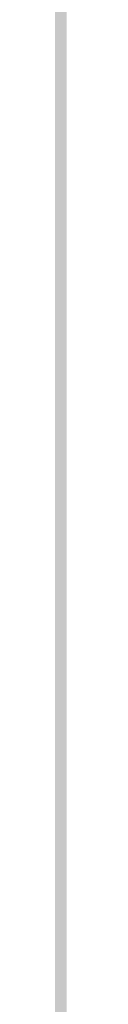
# Model space of a CAD drawing. Units: inches. Extents: x 2083 to 3317, y 1141 to 2115.
# Tile 201 of 256: x 3126.9579 to 3126.959, y 1263.6134 to 1264.1307. Entities that reach past the tile are written whole.
import ezdxf

# ---------------------------------------------------------------- set-up
doc = ezdxf.new("R2010")
doc.units = ezdxf.units.IN
doc.layers.add('A-ANNO-DIMS', color=2, linetype='Continuous', lineweight=18)
doc.layers.add('A-WALL-PATT', color=251, linetype='Continuous', lineweight=13, true_color=0x636466)
doc.styles.get("Standard").update_dxf_attribs({"font": 'arial.ttf'})
doc.dimstyles.new('ISO-25', dxfattribs={"dimtxt": 12, "dimasz": 12, "dimexe": 1.25, "dimexo": 0.625, "dimtad": 1, "dimlunit": 3, "dimtxsty": 'Standard', "dimcen": 2.5, "dimadec": 0, "dimazin": 0, "dimtfac": 1, "dimtmove": 0, "dimatfit": 3, "dimfxl": 1, "dimarcsym": 0})

# ---------------------------------------------------------------- blocks, each defined once
blk = doc.blocks.new('*D26')
at = {"layer": 'A-ANNO-DIMS', "color": 0, "lineweight": -2, "transparency": 16777216}
for p, q in [((3088.98584, 1274.91509), (3088.98584, 1270.95196)), ((3111.24004, 1274.91509), (3111.24004, 1270.95196)), ((3076.98584, 1272.20196), (2840.26245, 1272.20196)), ((3111.24004, 1272.20196), (3088.98584, 1272.20196)), ((3123.24004, 1272.20196), (3135.24004, 1272.20196))]:
    blk.add_line(p, q, dxfattribs=at)
at = {"layer": 'A-ANNO-DIMS', "color": 0, "transparency": 16777216}
for points in [[(3076.98584, 1274.20196), (3076.98584, 1270.20196), (3088.98584, 1272.20196)], [(3123.24004, 1274.20196), (3123.24004, 1270.20196), (3111.24004, 1272.20196)]]:
    blk.add_solid(points, dxfattribs=at)
at = {"layer": 'Defpoints', "color": 0, "transparency": 16777216}
for p in [(3088.98584, 1275.54009), (3111.24004, 1275.54009), (3088.98584, 1272.20196)]:
    blk.add_point(p, dxfattribs=at)
at = {"layer": 'A-ANNO-DIMS', "color": 0, "transparency": 16777216, "insert": (2952.62415, 1279.0316), "char_height": 12, "attachment_point": 5}
blk.add_mtext('NIGHTSTAND 1\'-10 1/2" TYP.', dxfattribs=at)
blk = doc.blocks.new('*D27')
at = {"layer": 'A-ANNO-DIMS', "color": 0, "lineweight": -2, "transparency": 16777216}
for p, q in [((3114.57817, 1309.79428), (3114.57817, 1321.79428)), ((3111.86504, 1297.79428), (3115.82817, 1297.79428)), ((3114.57817, 1297.79428), (3114.57817, 1275.54009)), ((3111.86504, 1275.54009), (3115.82817, 1275.54009)), ((3114.57817, 1263.54009), (3114.57817, 1140.98859))]:
    blk.add_line(p, q, dxfattribs=at)
at = {"layer": 'A-ANNO-DIMS', "color": 0, "transparency": 16777216}
for points in [[(3112.57817, 1309.79428), (3116.57817, 1309.79428), (3114.57817, 1297.79428)], [(3112.57817, 1263.54009), (3116.57817, 1263.54009), (3114.57817, 1275.54009)]]:
    blk.add_solid(points, dxfattribs=at)
at = {"layer": 'Defpoints', "color": 0, "transparency": 16777216}
for p in [(3111.24004, 1297.79428), (3111.24004, 1275.54009), (3114.57817, 1275.54009)]:
    blk.add_point(p, dxfattribs=at)
at = {"layer": 'A-ANNO-DIMS', "color": 0, "transparency": 16777216, "insert": (3107.74853, 1196.26434), "char_height": 12, "attachment_point": 5, "rotation": 90}
blk.add_mtext('1\'-10 1/2" TYP.', dxfattribs=at)

msp = doc.modelspace()

# ---------------------------------------------------------------- hatches: boundary and pattern name
at = {"layer": 'A-WALL-PATT'}
h = msp.add_hatch(color=256, dxfattribs=at)
h.dxf.hatch_style = 1
h.paths.add_polyline_path([(3126.95978, 2020.76136), (2748.95978, 2020.76136), (2604.95978, 2020.76136), (2226.95978, 2020.76136), (2226.95978, 1702.76136), (2466.95978, 1702.76136), (2466.95978, 1582.76136), (2418.95978, 1582.76136), (2418.95978, 1477.76136), (2226.95978, 1477.76136), (2226.95978, 1263.26136), (2544.95978, 1263.26136), (2544.95978, 1411.76136), (2604.95978, 1411.76136), (2685.95978, 1411.76136), (2685.95978, 1420.76136), (2604.95978, 1420.76136), (2604.95978, 1573.76136), (2604.95978, 1702.76136), (2604.95978, 2011.76136), (2748.95978, 2011.76136), (2748.95978, 1702.76136), (2862.95978, 1702.76136), (2862.95978, 1621.76136), (2871.95978, 1621.76136), (2871.95978, 1702.76136), (2883.95978, 1702.76136), (2883.95978, 1706.93946, -0.026459), (2883.95978, 1711.76136), (2757.95978, 1711.76136), (2757.95978, 1807.76136), (2787.95978, 1807.76136), (2787.95978, 1812.26136), (2757.95978, 1812.26136), (2757.95978, 2011.76136), (2877.95978, 2011.76136), (2877.95978, 1812.26136), (2847.95978, 1812.26136), (2847.95978, 1807.76136), (2889.83574, 1807.76136), (2889.83574, 1812.26136), (2882.45978, 1812.26136), (2882.45978, 2011.76136), (3117.95978, 2011.76136), (3117.95978, 1812.26136), (2937.83574, 1812.26136), (2937.83574, 1807.76136), (2995.70978, 1807.76136), (2995.70978, 1796.11767), (3000.20978, 1796.11767), (3000.20978, 1807.76136), (3117.95978, 1807.76136), (3117.95978, 1711.76136), (3000.20978, 1711.76136), (3000.20978, 1760.11767), (2998.5727, 1760.11767, -0.020711), (2995.70978, 1760.11767), (2995.70978, 1711.76136), (2931.95978, 1711.76136), (2931.95978, 1702.76136), (3126.95978, 1702.76136)])
h.paths.add_polyline_path([(2471.45978, 2011.76136), (2471.45978, 1810.01136), (2462.71694, 1810.01136), (2462.71694, 1805.51136), (2505.95978, 1805.51136), (2505.95978, 1810.01136), (2475.95978, 1810.01136), (2475.95978, 2011.76136), (2595.95978, 2011.76136), (2595.95978, 1810.01136), (2565.95978, 1810.01136), (2565.95978, 1805.51136), (2595.95978, 1805.51136), (2595.95978, 1711.76136), (2235.95978, 1711.76136), (2235.95978, 1805.51136), (2353.70978, 1805.51136), (2353.70978, 1796.05416), (2358.20978, 1796.05416), (2358.20978, 1805.51136), (2414.71694, 1805.51136), (2414.71694, 1810.01136), (2235.95978, 1810.01136), (2235.95978, 2011.76136)], flags=16)
h.paths.add_polyline_path([(2270.20473, 1994.61001), (2270.20473, 1970.61001), (2246.20473, 1970.61001), (2246.20473, 1994.61001)], flags=0)
edge = h.paths.add_edge_path(flags=0)
edge.add_ellipse((2332.02739, 1899.79818), major_axis=(-3.04299, 3.04299), ratio=0.1682525, start_angle=-161.33217, end_angle=-156.30711, ccw=False)
edge.add_ellipse((2333.08204, 1898.74353), major_axis=(-1.05465, 1.05465), ratio=0.4535321, start_angle=-123.37102, end_angle=-94.15911)
edge = h.paths.add_edge_path(flags=0)
edge.add_ellipse((2332.02739, 1968.87629), major_axis=(3.04299, 3.04299), ratio=0.1682525, start_angle=18.66783, end_angle=23.69289)
edge.add_spline(control_points=[(2332.9256, 1970.6911), (2332.22677, 1970.3361), (2330.89371, 1969.65891), (2328.41308, 1970.93214), (2327.20393, 1967.74871), (2324.7096, 1969.95559), (2322.53282, 1967.01235), (2320.01285, 1971.29581), (2317.68031, 1968.15784), (2316.04053, 1967.10205), (2315.4269, 1966.8096)], knot_values=[0, 0, 0, 0, 2.267059, 4.324559, 6.685584, 8.878641, 11.121502, 14.300359, 17.755284, 19.732645, 19.732645, 19.732645, 19.732645], degree=3, periodic=0)
edge.add_ellipse((2332.02739, 1968.87629), major_axis=(3.04299, 3.04299), ratio=0.1682525, start_angle=18.66783, end_angle=23.69289, ccw=False)
edge.add_ellipse((2333.08204, 1969.93094), major_axis=(1.05465, 1.05465), ratio=0.4535321, start_angle=56.62898, end_angle=85.84089, ccw=False)
edge = h.paths.add_edge_path(flags=0)
edge.add_spline(control_points=[(2296.42829, 1967.98791), (2293.6278, 1965.33631), (2287.70362, 1959.72709), (2299.74386, 1949.9957), (2294.53259, 1935.66853), (2290.57323, 1920.60351), (2293.39412, 1909.97369), (2296.18541, 1904.96654)], knot_values=[0.099185, 0.099185, 0.099185, 0.099185, 0.345301, 0.619822, 0.982653, 1.386093, 1.810555, 1.810555, 1.810555, 1.810555], degree=3, periodic=0)
edge.add_spline(control_points=[(2296.18541, 1904.96654), (2297.38358, 1902.6193), (2298.00097, 1901.94931), (2298.55297, 1901.46815)], knot_values=[0.006246, 0.006246, 0.006246, 0.006246, 0.055476, 0.055476, 0.055476, 0.055476], degree=3, periodic=0)
edge.add_spline(control_points=[(2298.55297, 1901.46815), (2297.25861, 1900.92322), (2295.22529, 1900.23213), (2293.06023, 1900.61421), (2292.10142, 1900.78841), (2292.08958, 1900.79057)], knot_values=[0.312835, 0.312835, 0.312835, 0.312835, 0.40178, 0.474987, 0.475903, 0.475903, 0.475903, 0.475903], degree=3, periodic=0)
edge.add_arc((2292.79365, 1904.66411), 3.93701, 215.4209, 259.69818, ccw=False)
edge.add_spline(control_points=[(2289.58531, 1902.3823), (2289.47665, 1902.53509), (2289.36848, 1902.68804), (2289.26086, 1902.84117)], knot_values=[0.102872, 0.102872, 0.102872, 0.102872, 0.116896, 0.116896, 0.116896, 0.116896], degree=3, periodic=0)
edge.add_spline(control_points=[(2289.26086, 1902.84117), (2288.6866, 1902.55019), (2287.64005, 1902.0199), (2285.88134, 1901.87395), (2283.85297, 1901.50435), (2281.71999, 1899.71054), (2278.46699, 1899.49294), (2276.15714, 1901.8832), (2272.25895, 1899.80407), (2267.77761, 1901.84318), (2262.24388, 1900.18403), (2257.41493, 1901.78206), (2254.31837, 1900.72612), (2253.17828, 1900.33734)], knot_values=[0, 0, 0, 0, 1.907977, 3.477176, 5.261074, 7.972851, 11.680248, 13.717921, 16.939592, 22.789562, 27.502503, 33.595215, 37.145618, 37.145618, 37.145618, 37.145618], degree=3, periodic=0)
edge.add_line((2253.17828, 1900.33734), (2250.24424, 1902.84117))
edge.add_line((2250.24424, 1902.84117), (2250.24424, 1965.8333))
edge.add_line((2250.24424, 1965.8333), (2253.17828, 1968.33712))
edge.add_spline(control_points=[(2253.17828, 1968.33712), (2254.31837, 1967.94835), (2257.41493, 1966.89241), (2262.24388, 1968.49043), (2267.77761, 1966.83128), (2271.52673, 1968.53722), (2273.87591, 1967.82829), (2274.2067, 1967.72764)], knot_values=[0, 0, 0, 0, 0.09018, 0.244935, 0.364644, 0.513233, 0.537855, 0.537855, 0.537855, 0.537855], degree=3, periodic=0)
edge.add_arc((2274.35289, 1963.79335), 3.93701, 72.05113, 92.12795, ccw=False)
edge.add_arc((2281.29693, 1985.23), 18.5963, 252.051134, 288.565722)
edge.add_arc((2292.31672, 1956.02888), 12.64608, 71.026788, 113.778218, ccw=False)
edge = h.paths.add_edge_path(flags=0)
edge.add_spline(control_points=[(2274.89941, 1951.85619), (2275.06616, 1951.61659), (2275.23269, 1951.37659), (2275.39799, 1951.13585)], knot_values=[1.409916, 1.409916, 1.409916, 1.409916, 1.43159, 1.43159, 1.43159, 1.43159], degree=3, periodic=0)
edge.add_spline(control_points=[(2275.39799, 1951.13585), (2275.79211, 1950.56189), (2276.17923, 1949.98377), (2276.54555, 1949.3971)], knot_values=[1.358238, 1.358238, 1.358238, 1.358238, 1.409916, 1.409916, 1.409916, 1.409916], degree=3, periodic=0)
edge.add_line((2276.54555, 1949.3971), (2277.43729, 1947.86218))
edge.add_spline(control_points=[(2277.43729, 1947.86218), (2276.30383, 1945.67311), (2274.6397, 1942.42688), (2274.63161, 1938.0939), (2272.79912, 1930.85155), (2274.35643, 1943.89705), (2275.94768, 1947.92336), (2276.54555, 1949.3971)], knot_values=[0.005632, 0.005632, 0.005632, 0.005632, 0.186014, 0.266002, 0.357087, 0.59639, 0.739732, 0.739732, 0.739732, 0.739732], degree=3, periodic=0)
edge.add_spline(control_points=[(2276.54555, 1949.3971), (2276.17923, 1949.98377), (2275.79211, 1950.56189), (2275.39799, 1951.13585)], knot_values=[1.358238, 1.358238, 1.358238, 1.358238, 1.409916, 1.409916, 1.409916, 1.409916], degree=3, periodic=0)
edge.add_spline(control_points=[(2275.39799, 1951.13585), (2274.9425, 1950.08045), (2274.20776, 1948.02527), (2273.9346, 1944.85148), (2272.46853, 1937.62749), (2273.46622, 1945.69647), (2274.70062, 1951.05947), (2274.89941, 1951.85619)], knot_values=[0.104364, 0.104364, 0.104364, 0.104364, 0.189636, 0.269624, 0.36071, 0.600013, 0.644622, 0.644622, 0.644622, 0.644622], degree=3, periodic=0)
h.paths.add_polyline_path([(2269.16751, 1963.12757, -0.357527), (2268.17063, 1960.97637, -0.092561), (2268.17063, 1939.43632, -0.357527), (2269.16751, 1937.28512, -0.357527), (2267.01631, 1938.282, -0.164785), (2254.68558, 1938.282, -0.357527), (2252.53438, 1937.28512, -0.357527), (2253.53126, 1939.43632, -0.092561), (2253.53126, 1960.97637, -0.357527), (2252.53438, 1963.12757, -0.357527), (2254.68558, 1962.13069, -0.164785), (2267.01631, 1962.13069, -0.357527)], flags=0)
h.paths.add_polyline_path([(2248.87407, 1967.8018), (2248.87407, 1957.02771), (2249.45778, 1957.02771), (2249.45778, 1911.64676), (2248.87407, 1911.64676), (2248.87407, 1900.87267), (2246.51186, 1900.87267, 0.197327), (2244.14966, 1902.45687), (2244.14966, 1966.21759, 0.197327), (2246.51186, 1967.8018)], flags=0)
h.paths.add_polyline_path([(2269.16751, 1931.38934, -0.357527), (2268.17063, 1929.23814, -0.092561), (2268.17063, 1907.6981, -0.357527), (2269.16751, 1905.54689, -0.357527), (2267.01631, 1906.54377, -0.164785), (2254.68558, 1906.54377, -0.357527), (2252.53438, 1905.54689, -0.357527), (2253.53126, 1907.6981, -0.092561), (2253.53126, 1929.23814, -0.357527), (2252.53438, 1931.38934, -0.357527), (2254.68558, 1930.39246, -0.164785), (2267.01631, 1930.39246, -0.357527)], flags=0)
edge = h.paths.add_edge_path(flags=0)
edge.add_spline(control_points=[(2276.19686, 1906.7237), (2276.16814, 1909.02893), (2276.11405, 1913.37185), (2270.59842, 1924.92498), (2273.90517, 1919.01278), (2275.92171, 1916.26206), (2275.47457, 1912.40215), (2277.25787, 1910.38062), (2276.69604, 1908.22504), (2276.64622, 1906.81302), (2276.61782, 1906.00841)], knot_values=[0, 0, 0, 0, 8.61026, 16.221274, 18.843057, 23.804898, 27.440828, 29.356102, 31.203478, 33.650687, 33.650687, 33.650687, 33.650687], degree=3, periodic=0)
edge.add_spline(control_points=[(2276.61782, 1906.00841), (2276.62331, 1905.62414), (2276.49774, 1904.62866), (2275.44178, 1903.85473), (2274.93731, 1903.08045), (2274.85908, 1902.84117)], knot_values=[0.156488, 0.156488, 0.156488, 0.156488, 0.184398, 0.231376, 0.250598, 0.250598, 0.250598, 0.250598], degree=3, periodic=0)
edge.add_line((2274.85908, 1902.84117), (2276.50598, 1902.84117))
edge.add_spline(control_points=[(2276.50598, 1902.84117), (2276.78831, 1903.08494), (2277.66507, 1904.1252), (2278.24954, 1904.34074), (2277.65387, 1908.52739), (2278.15567, 1906.22781), (2278.10046, 1905.28595), (2278.84667, 1904.06901), (2277.85679, 1903.41495), (2277.87419, 1902.99105), (2277.90356, 1902.84117)], knot_values=[0.059574, 0.059574, 0.059574, 0.059574, 0.080753, 0.103741, 0.16972, 0.176036, 0.207137, 0.240474, 0.262341, 0.27366, 0.27366, 0.27366, 0.27366], degree=3, periodic=0)
edge.add_line((2277.90356, 1902.84117), (2280.02983, 1902.84117))
edge.add_spline(control_points=[(2280.02983, 1902.84117), (2279.88822, 1903.0884), (2279.49926, 1903.98155), (2280.15228, 1905.93935), (2278.10362, 1909.65776), (2279.76239, 1907.18529), (2280.3279, 1904.87486), (2280.48511, 1903.48959), (2281.46327, 1903.24943), (2281.75834, 1902.9365), (2281.83404, 1902.84117)], knot_values=[0.013856, 0.013856, 0.013856, 0.013856, 0.034874, 0.088867, 0.107879, 0.126738, 0.158714, 0.193757, 0.217487, 0.226722, 0.226722, 0.226722, 0.226722], degree=3, periodic=0)
edge.add_spline(control_points=[(2281.83404, 1902.84117), (2281.78753, 1902.8267), (2281.64702, 1902.78299), (2281.39553, 1902.85949), (2281.08808, 1902.98524), (2280.72068, 1903.0609), (2280.33345, 1903.02573), (2280.12477, 1902.89888), (2280.02983, 1902.84117)], knot_values=[0, 0, 0, 0, 0.14413, 0.435517, 0.749276, 1.153046, 1.548371, 1.878348, 1.878348, 1.878348, 1.878348], degree=3, periodic=0)
edge.add_line((2280.02983, 1902.84117), (2277.90356, 1902.84117))
edge.add_spline(control_points=[(2277.90356, 1902.84117), (2277.89286, 1902.79586), (2277.8654, 1902.67964), (2277.60748, 1902.68748), (2277.27405, 1902.8007), (2276.83792, 1902.61977), (2276.58381, 1902.78926), (2276.50598, 1902.84117)], knot_values=[0, 0, 0, 0, 0.127189, 0.326199, 0.628009, 1.24357, 1.515331, 1.515331, 1.515331, 1.515331], degree=3, periodic=0)
edge.add_line((2276.50598, 1902.84117), (2274.85908, 1902.84117))
edge.add_spline(control_points=[(2274.85908, 1902.84117), (2274.81444, 1902.89859), (2274.72513, 1903.01345), (2274.49348, 1903.11897), (2274.24429, 1902.96054), (2273.93712, 1903.18494), (2273.61404, 1902.98314), (2273.40832, 1902.88304), (2273.32225, 1902.84117)], knot_values=[0, 0, 0, 0, 0.21843, 0.436957, 0.687977, 0.990379, 1.398396, 1.69185, 1.69185, 1.69185, 1.69185], degree=3, periodic=0)
edge.add_spline(control_points=[(2273.32225, 1902.84117), (2273.61674, 1903.44569), (2274.274, 1904.53825), (2276.02724, 1904.5737), (2276.20696, 1906.58364), (2276.19686, 1906.7237)], knot_values=[0.012227, 0.012227, 0.012227, 0.012227, 0.059472, 0.106218, 0.134458, 0.134458, 0.134458, 0.134458], degree=3, periodic=0)
h.paths.add_polyline_path([(2270.77605, 1897.78983), (2270.77605, 1873.78983), (2246.77605, 1873.78983), (2246.77605, 1897.78983)], flags=0)
h.paths.add_polyline_path([(2353.70978, 1760.00506), (2353.70978, 1760.05416), (2358.20978, 1760.05416, -0.033729)], flags=0)
h.paths.add_polyline_path([(2321.81912, 1737.52919), (2341.99533, 1737.52919, -0.414214), (2343.20327, 1736.32124), (2343.20327, 1721.0206, -0.414214), (2341.99533, 1719.81265), (2321.81912, 1719.81265, -0.414214), (2320.61117, 1721.0206), (2320.61117, 1736.32124, -0.414214)], flags=0)
h.paths.add_polyline_path([(2324.23501, 1736.32124), (2339.57944, 1736.32124, -0.414214), (2341.99533, 1733.90535), (2341.99533, 1725.44973, -0.414214), (2339.57944, 1723.03384), (2333.68059, 1723.03384), (2333.84532, 1722.04547, -0.870646), (2335.4254, 1721.82589, -0.767327), (2333.92269, 1721.42324), (2331.29102, 1721.42324, -0.767327), (2329.78832, 1721.82589, -0.870646), (2331.3684, 1722.04547), (2331.53313, 1723.03384), (2324.23501, 1723.03384, -0.414214), (2321.81912, 1725.44973), (2321.81912, 1733.90535, -0.414214)], flags=0)
h.paths.add_polyline_path([(2570.48379, 1928.61544), (2589.68379, 1928.61544), (2590.16883, 1928.61544), (2590.16883, 1904.9934), (2570.48379, 1904.9934)], flags=0)
h.paths.add_polyline_path([(2574.44732, 1927.26382, -1), (2572.82884, 1927.26382, -1)], flags=0)
h.paths.add_polyline_path([(2573.08987, 1926.94088), (2573.92503, 1927.77604), (2574.14774, 1927.55333), (2573.31258, 1926.71817)], flags=0)
h.paths.add_polyline_path([(2578.77906, 1919.72962, -1), (2571.59166, 1919.72962, -1)], flags=0)
h.paths.add_polyline_path([(2578.38536, 1919.72962, -1), (2571.98536, 1919.72962, -1)], flags=0)
h.paths.add_polyline_path([(2331.59576, 1729.47622, -1), (2333.61795, 1729.47622, -1)], flags=0)
h.paths.add_polyline_path([(2578.03423, 1927.26382, -1), (2576.41574, 1927.26382, -1)], flags=0)
h.paths.add_polyline_path([(2576.68885, 1927.53109), (2576.91156, 1927.7538), (2577.74673, 1926.91863), (2577.52402, 1926.69592)], flags=0)
h.paths.add_polyline_path([(2578.13906, 1909.85954, -1), (2572.23166, 1909.85954, -1)], flags=0)
h.paths.add_polyline_path([(2577.74536, 1909.85954, -1), (2572.62536, 1909.85954, -1)], flags=0)
h.paths.add_polyline_path([(2583.79772, 1927.26382, -1), (2582.17923, 1927.26382, -1)], flags=0)
h.paths.add_polyline_path([(2582.71865, 1927.7538), (2583.55381, 1926.91863), (2583.3311, 1926.69592), (2582.49594, 1927.53109)], flags=0)
h.paths.add_polyline_path([(2582.49594, 1927.53109), (2582.71865, 1927.7538), (2583.55381, 1926.91863), (2583.3311, 1926.69592)], flags=0)
h.paths.add_polyline_path([(2587.73906, 1920.52962, -1), (2581.83166, 1920.52962, -1)], flags=0)
h.paths.add_polyline_path([(2587.34536, 1920.52962, -1), (2582.22536, 1920.52962, -1)], flags=0)
h.paths.add_polyline_path([(2587.38462, 1927.26382, -1), (2585.76613, 1927.26382, -1)], flags=0)
h.paths.add_polyline_path([(2586.08199, 1926.98025), (2586.91716, 1927.81541), (2587.13987, 1927.5927), (2586.3047, 1926.75754)], flags=0)
h.paths.add_polyline_path([(2588.37906, 1910.65954, -1), (2581.19166, 1910.65954, -1)], flags=0)
h.paths.add_polyline_path([(2587.98536, 1910.65954, -1), (2581.58536, 1910.65954, -1)], flags=0)
h.paths.add_polyline_path([(2417.16773, 1729.4779), (2437.34394, 1729.4779, -0.414214), (2438.55188, 1728.26995), (2438.55188, 1712.96931, -0.414214), (2437.34394, 1711.76136), (2417.16773, 1711.76136, -0.414214), (2415.95978, 1712.96931), (2415.95978, 1728.26995, -0.414214)], flags=0)
h.paths.add_polyline_path([(2419.58362, 1728.26995), (2434.92805, 1728.26995, -0.414214), (2437.34394, 1725.85406), (2437.34394, 1717.39844, -0.414214), (2434.92805, 1714.98255), (2429.0292, 1714.98255), (2429.19393, 1713.99418, -0.870646), (2430.77401, 1713.7746, -0.767327), (2429.2713, 1713.37195), (2426.63963, 1713.37195, -0.767327), (2425.13693, 1713.7746, -0.870646), (2426.71701, 1713.99418), (2426.88174, 1714.98255), (2419.58362, 1714.98255, -0.414214), (2417.16773, 1717.39844), (2417.16773, 1725.85406, -0.414214)], flags=0)
h.paths.add_polyline_path([(2419.58362, 1728.26995), (2434.92805, 1728.26995, -0.414214), (2437.34394, 1725.85406), (2437.34394, 1717.39844, -0.414214), (2434.92805, 1714.98255), (2429.0292, 1714.98255), (2428.35812, 1719.00903), (2427.55282, 1719.00903), (2426.88174, 1714.98255), (2419.58362, 1714.98255, -0.414214), (2417.16773, 1717.39844), (2417.16773, 1725.85406, -0.414214)], flags=0)
h.paths.add_polyline_path([(2426.94437, 1721.42492, -1), (2428.96656, 1721.42492, -1)], flags=0)
h.paths.add_polyline_path([(2475.95978, 1702.76136), (2595.95978, 1702.76136), (2595.95978, 1582.76136), (2475.95978, 1582.76136)], flags=16)
h.paths.add_polyline_path([(2427.95978, 1573.76136), (2595.95978, 1573.76136), (2595.95978, 1468.76136), (2595.95978, 1420.76136), (2384.45978, 1420.76136), (2384.45978, 1468.76136), (2427.95978, 1468.76136)], flags=16)
h.paths.add_polyline_path([(2379.95978, 1468.76136), (2379.95978, 1420.76136), (2235.95978, 1420.76136), (2235.95978, 1468.76136)], flags=16)
h.paths.add_polyline_path([(2317.816, 1466.69577), (2337.9922, 1466.69577, -0.414214), (2339.20015, 1465.48782), (2339.20015, 1450.18718, -0.414214), (2337.9922, 1448.97923), (2317.816, 1448.97923, -0.414214), (2316.60805, 1450.18718), (2316.60805, 1465.48782, -0.414214)], flags=0)
h.paths.add_polyline_path([(2320.23189, 1465.48782), (2335.57631, 1465.48782, -0.414214), (2337.9922, 1463.07193), (2337.9922, 1454.61631, -0.414214), (2335.57631, 1452.20042), (2329.67747, 1452.20042), (2329.84219, 1451.21205, -0.870646), (2331.42228, 1450.99247, -0.767327), (2329.91957, 1450.58983), (2327.2879, 1450.58983, -0.767327), (2325.7852, 1450.99247, -0.870646), (2327.36528, 1451.21205), (2327.53001, 1452.20042), (2320.23189, 1452.20042, -0.414214), (2317.816, 1454.61631), (2317.816, 1463.07193, -0.414214)], flags=0)
h.paths.add_polyline_path([(2320.23189, 1465.48782), (2335.57631, 1465.48782, -0.414214), (2337.9922, 1463.07193), (2337.9922, 1454.61631, -0.414214), (2335.57631, 1452.20042), (2329.67747, 1452.20042), (2329.00638, 1456.22691), (2328.20109, 1456.22691), (2327.53001, 1452.20042), (2320.23189, 1452.20042, -0.414214), (2317.816, 1454.61631), (2317.816, 1463.07193, -0.414214)], flags=0)
h.paths.add_polyline_path([(2327.59264, 1458.6428, -1), (2329.61483, 1458.6428, -1)], flags=0)
h.paths.add_polyline_path([(2244.41174, 1433.34045), (2241.92094, 1433.34045, -0.414214), (2240.01786, 1435.24354), (2240.01786, 1440.95281, -0.414211), (2241.92093, 1442.8559), (2244.41174, 1442.8559, -1.976472)], flags=0)
h.paths.add_polyline_path([(2245.35689, 1434.39754, -0.414214), (2245.35689, 1441.79881, -2.144098)], flags=0)
h.paths.add_polyline_path([(2535.95978, 1416.26136), (2535.95978, 1272.26136), (2235.95978, 1272.26136), (2235.95978, 1416.26136)], flags=16)
h.paths.add_polyline_path([(2260.11956, 1384.29284), (2260.11956, 1362.03865), (2237.86537, 1362.03865), (2237.86537, 1384.29284)], flags=0)
edge = h.paths.add_edge_path(flags=0)
edge.add_line((2318.25185, 1362.0933), (2318.1458, 1362.00097))
edge.add_ellipse((2317.44512, 1360.43104), major_axis=(2.82164, 2.82164), ratio=0.1682525, start_angle=18.66783, end_angle=20.94813, ccw=False)
edge.add_ellipse((2318.42305, 1361.40897), major_axis=(0.97793, 0.97793), ratio=0.4535321, start_angle=56.62898, end_angle=70.2262, ccw=False)
edge = h.paths.add_edge_path(flags=0)
edge.add_line((2319.10737, 1295.57108), (2319.01504, 1295.67713))
edge.add_ellipse((2317.44512, 1296.37781), major_axis=(-2.82164, 2.82164), ratio=0.1682525, start_angle=-161.33217, end_angle=-159.05187, ccw=False)
edge.add_ellipse((2318.42305, 1295.39988), major_axis=(-0.97793, 0.97793), ratio=0.4535321, start_angle=-123.37102, end_angle=-109.7738)
edge = h.paths.add_edge_path(flags=0)
edge.add_spline(control_points=[(2284.21035, 1301.17022), (2284.58069, 1300.44472), (2284.89119, 1299.89202), (2285.15955, 1299.46102)], knot_values=[0.039066, 0.039066, 0.039066, 0.039066, 0.055476, 0.055476, 0.055476, 0.055476], degree=3, periodic=0)
edge.add_line((2285.15955, 1299.46102), (2284.21035, 1301.17022))
edge = h.paths.add_edge_path(flags=0)
edge.add_line((2280.41246, 1297.29801), (2283.36999, 1297.03612))
edge.add_line((2283.36999, 1297.03612), (2286.40569, 1297.92631))
edge.add_spline(control_points=[(2286.40569, 1297.92631), (2285.30549, 1297.46312), (2284.34478, 1297.12915), (2283.36999, 1297.03612)], knot_values=[0.394369, 0.394369, 0.394369, 0.394369, 0.475903, 0.475903, 0.475903, 0.475903], degree=3, periodic=0)
edge.add_spline(control_points=[(2283.36999, 1297.03612), (2283.28139, 1297.02767), (2282.31629, 1296.95734), (2281.3125, 1297.13448), (2280.42344, 1297.29602), (2280.41246, 1297.29801)], knot_values=[0.312835, 0.312835, 0.312835, 0.312835, 0.320246, 0.393453, 0.394369, 0.394369, 0.394369, 0.394369], degree=3, periodic=0)
edge = h.paths.add_edge_path(flags=0)
edge.add_line((2284.43556, 1359.60729), (2280.44629, 1355.32805))
edge.add_line((2280.44629, 1355.32805), (2279.57999, 1351.01775))
edge.add_line((2279.57999, 1351.01775), (2282.41297, 1346.58043))
edge.add_spline(control_points=[(2282.41297, 1346.58043), (2283.15333, 1345.58924), (2284.2529, 1344.0289), (2284.80104, 1342.38717), (2284.93516, 1341.80554)], knot_values=[1.240098, 1.240098, 1.240098, 1.240098, 1.332892, 1.382712, 1.382712, 1.382712, 1.382712], degree=3, periodic=0)
edge.add_spline(control_points=[(2284.93516, 1341.80554), (2285.31911, 1340.1406), (2285.23303, 1338.4092), (2284.90994, 1336.65412)], knot_values=[1.097484, 1.097484, 1.097484, 1.097484, 1.240098, 1.240098, 1.240098, 1.240098], degree=3, periodic=0)
edge.add_spline(control_points=[(2284.90994, 1336.65412), (2284.58685, 1334.89904), (2284.02675, 1333.12027), (2283.46264, 1331.36058)], knot_values=[0.95487, 0.95487, 0.95487, 0.95487, 1.097484, 1.097484, 1.097484, 1.097484], degree=3, periodic=0)
edge.add_line((2283.46264, 1331.36058), (2281.89038, 1326.15336))
edge.add_line((2281.89038, 1326.15336), (2280.75626, 1321.05609))
edge.add_line((2280.75626, 1321.05609), (2280.2992, 1316.00198))
edge.add_line((2280.2992, 1316.00198), (2280.71593, 1310.95007))
edge.add_line((2280.71593, 1310.95007), (2282.02809, 1305.97214))
edge.add_line((2282.02809, 1305.97214), (2284.21035, 1301.17022))
edge.add_spline(control_points=[(2284.21035, 1301.17022), (2283.34073, 1302.73019), (2282.6119, 1304.33649), (2282.02809, 1305.97214)], knot_values=[0.099185, 0.099185, 0.099185, 0.099185, 0.241799, 0.241799, 0.241799, 0.241799], degree=3, periodic=0)
edge.add_spline(control_points=[(2282.02809, 1305.97214), (2281.44428, 1307.60778), (2281.00549, 1309.27276), (2280.71593, 1310.95007)], knot_values=[0.241799, 0.241799, 0.241799, 0.241799, 0.384413, 0.384413, 0.384413, 0.384413], degree=3, periodic=0)
edge.add_spline(control_points=[(2280.71593, 1310.95007), (2280.43324, 1312.58761), (2280.28939, 1314.27696), (2280.29889, 1315.96203), (2280.2992, 1316.00198)], knot_values=[0.384413, 0.384413, 0.384413, 0.384413, 0.523647, 0.527028, 0.527028, 0.527028, 0.527028], degree=3, periodic=0)
edge.add_spline(control_points=[(2280.2992, 1316.00198), (2280.31233, 1317.68696), (2280.47787, 1319.36793), (2280.75626, 1321.05609)], knot_values=[0.527028, 0.527028, 0.527028, 0.527028, 0.669642, 0.669642, 0.669642, 0.669642], degree=3, periodic=0)
edge.add_spline(control_points=[(2280.75626, 1321.05609), (2281.03465, 1322.74425), (2281.42588, 1324.43961), (2281.89038, 1326.15336)], knot_values=[0.669642, 0.669642, 0.669642, 0.669642, 0.812256, 0.812256, 0.812256, 0.812256], degree=3, periodic=0)
edge.add_spline(control_points=[(2281.89038, 1326.15336), (2282.26438, 1327.53325), (2282.78787, 1329.26181), (2283.35275, 1331.01778), (2283.46264, 1331.36058)], knot_values=[0.812256, 0.812256, 0.812256, 0.812256, 0.927087, 0.95487, 0.95487, 0.95487, 0.95487], degree=3, periodic=0)
edge.add_line((2283.46264, 1331.36058), (2284.90994, 1336.65412))
edge.add_line((2284.90994, 1336.65412), (2284.93516, 1341.80554))
edge.add_line((2284.93516, 1341.80554), (2282.41297, 1346.58043))
edge.add_spline(control_points=[(2282.41297, 1346.58043), (2281.27513, 1348.10379), (2280.07845, 1349.57032), (2279.57999, 1351.01775)], knot_values=[1.382712, 1.382712, 1.382712, 1.382712, 1.525326, 1.525326, 1.525326, 1.525326], degree=3, periodic=0)
edge.add_spline(control_points=[(2279.57999, 1351.01775), (2279.44328, 1351.41472), (2279.13631, 1352.85692), (2279.73519, 1354.29039), (2280.44629, 1355.32805)], knot_values=[1.525326, 1.525326, 1.525326, 1.525326, 1.564439, 1.667941, 1.667941, 1.667941, 1.667941], degree=3, periodic=0)
edge.add_spline(control_points=[(2280.44629, 1355.32805), (2281.42611, 1356.75784), (2282.93084, 1358.18256), (2284.43556, 1359.60729)], knot_values=[1.667941, 1.667941, 1.667941, 1.667941, 1.810555, 1.810555, 1.810555, 1.810555], degree=3, periodic=0)
edge.add_arc((2280.62307, 1348.51818), 11.72618, 71.026788, 113.778218)
edge.add_arc((2270.40489, 1375.59516), 17.24357, 252.051134, 288.565722, ccw=False)
edge.add_arc((2263.96597, 1355.71785), 3.65062, 72.05113, 92.12795)
edge.add_arc((2263.96597, 1355.71785), 3.65062, 92.12795, 177.98513)
edge.add_spline(control_points=[(2260.3176, 1355.8462), (2260.26042, 1354.22067), (2260.55128, 1350.18655), (2262.99934, 1346.76625), (2264.47274, 1344.64902)], knot_values=[1.43159, 1.43159, 1.43159, 1.43159, 1.564144, 1.770695, 1.770695, 1.770695, 1.770695], degree=3, periodic=0)
edge.add_line((2264.47274, 1344.64902), (2264.93559, 1343.98253))
edge.add_spline(control_points=[(2263.80104, 1340.24811), (2263.84324, 1340.51409), (2264.06724, 1341.75647), (2264.51269, 1343.00245), (2264.93505, 1343.98108)], knot_values=[0.53657, 0.53657, 0.53657, 0.53657, 0.559349, 0.644622, 0.644622, 0.644622, 0.644622], degree=3, periodic=0)
edge.add_spline(control_points=[(2264.93505, 1343.98108), (2265.11777, 1343.71497), (2265.29888, 1343.44791), (2265.47676, 1343.17936)], knot_values=[1.384077, 1.384077, 1.384077, 1.384077, 1.409916, 1.409916, 1.409916, 1.409916], degree=3, periodic=0)
edge.add_spline(control_points=[(2265.47676, 1343.17936), (2265.65464, 1342.91082), (2265.8293, 1342.64081), (2265.99913, 1342.36881)], knot_values=[1.358238, 1.358238, 1.358238, 1.358238, 1.384077, 1.384077, 1.384077, 1.384077], degree=3, periodic=0)
edge.add_line((2265.99913, 1342.36881), (2266.82601, 1340.94555))
edge.add_spline(control_points=[(2266.82601, 1340.94555), (2268.8944, 1337.08969), (2271.39817, 1325.843), (2270.51616, 1310.56856), (2275.91938, 1301.86061), (2277.78951, 1299.19945)], knot_values=[0.116896, 0.116896, 0.116896, 0.116896, 0.472987, 1.050969, 1.313793, 1.313793, 1.313793, 1.313793], degree=3, periodic=0)
edge.add_spline(control_points=[(2277.78951, 1299.19945), (2277.83941, 1299.12845), (2277.88943, 1299.0575), (2277.93957, 1298.98658)], knot_values=[0.109884, 0.109884, 0.109884, 0.109884, 0.116896, 0.116896, 0.116896, 0.116896], degree=3, periodic=0)
edge.add_line((2277.93957, 1298.98658), (2277.78885, 1299.19911))
edge.add_spline(control_points=[(2277.78885, 1299.19911), (2277.25658, 1298.92941), (2276.28635, 1298.4379), (2275.03935, 1298.33442), (2274.38333, 1298.2389), (2274.21525, 1298.20934)], knot_values=[33.12187, 33.12187, 33.12187, 33.12187, 35.029056, 36.598255, 37.144827, 37.144827, 37.144827, 37.144827], degree=3, periodic=0)
edge.add_line((2274.21525, 1298.20934), (2273.07315, 1297.89296))
edge.add_spline(control_points=[(2273.07315, 1297.89296), (2272.32294, 1297.57978), (2271.03915, 1296.51051), (2269.24839, 1296.22606), (2268.4231, 1296.37465)], knot_values=[26.532584, 26.532584, 26.532584, 26.532584, 29.198919, 31.839101, 31.839101, 31.839101, 31.839101], degree=3, periodic=0)
edge.add_line((2268.4231, 1296.37465), (2263.8785, 1297.45753))
edge.add_spline(control_points=[(2263.8785, 1297.45753), (2263.55608, 1297.35943), (2261.86031, 1296.83869), (2260.23878, 1297.28241), (2258.93345, 1297.51646)], knot_values=[15.919551, 15.919551, 15.919551, 15.919551, 16.939592, 21.226067, 21.226067, 21.226067, 21.226067], degree=3, periodic=0)
edge.add_line((2258.93345, 1297.51646), (2254.05523, 1297.32901))
edge.add_spline(control_points=[(2254.05523, 1297.32901), (2253.75553, 1297.29582), (2252.11368, 1297.16517), (2250.46187, 1297.54422), (2249.12969, 1297.66788)], knot_values=[5.306517, 5.306517, 5.306517, 5.306517, 6.276435, 10.613034, 10.613034, 10.613034, 10.613034], degree=3, periodic=0)
edge.add_line((2249.12969, 1297.66788), (2244.33165, 1296.87776))
edge.add_line((2244.33165, 1296.87776), (2241.61103, 1299.19945))
edge.add_line((2241.61103, 1299.19945), (2241.61103, 1357.6094))
edge.add_line((2241.61103, 1357.6094), (2244.33165, 1359.9311))
edge.add_line((2244.33165, 1359.9311), (2252.72882, 1359.54269))
edge.add_spline(control_points=[(2252.72882, 1359.54269), (2252.87094, 1359.54644), (2253.30574, 1359.54817), (2253.73984, 1359.51427), (2254.03174, 1359.48243)], knot_values=[0.233291, 0.233291, 0.233291, 0.233291, 0.244935, 0.268927, 0.268927, 0.268927, 0.268927], degree=3, periodic=0)
edge.add_line((2254.03174, 1359.48243), (2259.58719, 1359.41639))
edge.add_spline(control_points=[(2259.58719, 1359.41639), (2260.67707, 1359.6285), (2262.0732, 1359.897), (2263.52369, 1359.45928), (2263.83042, 1359.36595)], knot_values=[0.422516, 0.422516, 0.422516, 0.422516, 0.513233, 0.537855, 0.537855, 0.537855, 0.537855], degree=3, periodic=0)
edge.add_arc((2263.96597, 1355.71785), 3.65062, 72.05113, 92.12795, ccw=False)
edge.add_arc((2270.40489, 1375.59516), 17.24357, 252.051134, 288.565722)
edge.add_arc((2280.62307, 1348.51818), 11.72618, 71.026788, 113.778218, ccw=False)
h.paths.add_polyline_path([(2240.34053, 1359.43471), (2240.34053, 1349.44435), (2240.88178, 1349.44435), (2240.88178, 1307.3645), (2240.34053, 1307.3645), (2240.34053, 1297.37414), (2238.15016, 1297.37414, 0.197327), (2235.95978, 1298.84311), (2235.95978, 1357.96575, 0.197327), (2238.15016, 1359.43471)], flags=0)
h.paths.add_polyline_path([(2259.15779, 1355.1005, -0.357527), (2258.23342, 1353.10578, -0.092561), (2258.23342, 1333.1326, -0.357527), (2259.15779, 1331.13788, -0.357527), (2257.16307, 1332.06225, -0.164785), (2245.7293, 1332.06225, -0.357527), (2243.73458, 1331.13788, -0.357527), (2244.65895, 1333.1326, -0.092561), (2244.65895, 1353.10578, -0.357527), (2243.73458, 1355.1005, -0.357527), (2245.7293, 1354.17613, -0.164785), (2257.16307, 1354.17613, -0.357527)], flags=0)
edge = h.paths.add_edge_path(flags=0)
edge.add_line((2265.99913, 1342.36881), (2266.82601, 1340.94555))
edge.add_line((2266.82601, 1340.94555), (2265.30756, 1337.81407))
edge.add_line((2265.30756, 1337.81407), (2264.35823, 1334.65294))
edge.add_line((2264.35823, 1334.65294), (2264.26201, 1333.7997))
edge.add_spline(control_points=[(2264.26201, 1333.7997), (2264.20836, 1333.18705), (2264.16206, 1332.36553), (2264.00714, 1331.41393), (2263.96905, 1331.20183)], knot_values=[0.464444, 0.464444, 0.464444, 0.464444, 0.516691, 0.531608, 0.531608, 0.531608, 0.531608], degree=3, periodic=0)
edge.add_spline(control_points=[(2263.96905, 1331.20183), (2263.77453, 1330.11887), (2263.42437, 1328.79084), (2263.25742, 1328.53065), (2263.23403, 1328.51461)], knot_values=[0.372682, 0.372682, 0.372682, 0.372682, 0.44885, 0.464444, 0.464444, 0.464444, 0.464444], degree=3, periodic=0)
edge.add_spline(control_points=[(2263.23403, 1328.51461), (2263.09638, 1328.42023), (2263.13117, 1329.30148), (2263.27495, 1330.61575)], knot_values=[0.280919, 0.280919, 0.280919, 0.280919, 0.372682, 0.372682, 0.372682, 0.372682], degree=3, periodic=0)
edge.add_spline(control_points=[(2263.27495, 1330.61575), (2263.41874, 1331.93002), (2263.67152, 1333.67732), (2263.96985, 1335.31503)], knot_values=[0.189157, 0.189157, 0.189157, 0.189157, 0.280919, 0.280919, 0.280919, 0.280919], degree=3, periodic=0)
edge.add_spline(control_points=[(2263.96985, 1335.31503), (2264.1005, 1336.03219), (2264.41878, 1337.62191), (2264.75485, 1338.86443), (2264.94742, 1339.49112)], knot_values=[0.097394, 0.097394, 0.097394, 0.097394, 0.137578, 0.189157, 0.189157, 0.189157, 0.189157], degree=3, periodic=0)
edge.add_spline(control_points=[(2264.94742, 1339.49112), (2265.29002, 1340.60605), (2265.64424, 1341.494), (2265.99913, 1342.36881)], knot_values=[0.005632, 0.005632, 0.005632, 0.005632, 0.097394, 0.097394, 0.097394, 0.097394], degree=3, periodic=0)
h.paths.add_polyline_path([(2259.15779, 1325.67097, -0.357527), (2258.23342, 1323.67625, -0.092561), (2258.23342, 1303.70307, -0.357527), (2259.15779, 1301.70835, -0.357527), (2257.16307, 1302.63272, -0.164785), (2245.7293, 1302.63272, -0.357527), (2243.73458, 1301.70835, -0.357527), (2244.65895, 1303.70307, -0.092561), (2244.65895, 1323.67625, -0.357527), (2243.73458, 1325.67097, -0.357527), (2245.7293, 1324.74661, -0.164785), (2257.16307, 1324.74661, -0.357527)], flags=0)
edge = h.paths.add_edge_path(flags=0)
edge.add_spline(control_points=[(2261.70894, 1317.31142), (2261.67948, 1317.41758), (2261.76186, 1317.38853), (2262.49074, 1316.08987), (2262.96218, 1315.3009)], knot_values=[14.955861, 14.955861, 14.955861, 14.955861, 16.221274, 18.694826, 18.694826, 18.694826, 18.694826], degree=3, periodic=0)
edge.add_spline(control_points=[(2262.96218, 1315.3009), (2262.99044, 1315.25362), (2263.7021, 1314.06738), (2264.34898, 1313.12715), (2264.73005, 1312.16415)], knot_values=[18.694826, 18.694826, 18.694826, 18.694826, 18.843057, 22.433791, 22.433791, 22.433791, 22.433791], degree=3, periodic=0)
edge.add_spline(control_points=[(2264.73005, 1312.16415), (2264.87556, 1311.79644), (2265.17687, 1310.76981), (2265.14307, 1309.55926), (2265.24774, 1308.82419)], knot_values=[22.433791, 22.433791, 22.433791, 22.433791, 23.804898, 26.172756, 26.172756, 26.172756, 26.172756], degree=3, periodic=0)
edge.add_line((2265.24774, 1308.82419), (2265.85077, 1307.17189))
edge.add_spline(control_points=[(2265.85077, 1307.17189), (2266.06502, 1306.82168), (2266.38439, 1306.33225), (2266.4244, 1305.78055), (2266.42037, 1305.61122)], knot_values=[28.062562, 28.062562, 28.062562, 28.062562, 29.356102, 29.911721, 29.911721, 29.911721, 29.911721], degree=3, periodic=0)
edge.add_spline(control_points=[(2266.42037, 1305.61122), (2266.41612, 1305.43259), (2266.394, 1305.25), (2266.36478, 1305.06586)], knot_values=[29.911721, 29.911721, 29.911721, 29.911721, 30.497837, 30.497837, 30.497837, 30.497837], degree=3, periodic=0)
edge.add_line((2266.36478, 1305.06586), (2266.06615, 1302.1363))
edge.add_spline(control_points=[(2266.06615, 1302.1363), (2266.07124, 1301.77998), (2265.99808, 1301.19998), (2265.66327, 1300.75896), (2265.50891, 1300.58588)], knot_values=[0.156488, 0.156488, 0.156488, 0.156488, 0.184398, 0.203543, 0.203543, 0.203543, 0.203543], degree=3, periodic=0)
edge.add_line((2265.50891, 1300.58588), (2264.43534, 1299.19945))
edge.add_line((2264.43534, 1299.19945), (2265.96244, 1299.19945))
edge.add_line((2265.96244, 1299.19945), (2267.33599, 1301.17528))
edge.add_line((2267.33599, 1301.17528), (2267.31167, 1301.98624))
edge.add_spline(control_points=[(2267.31167, 1301.98624), (2267.26111, 1302.8624), (2267.16021, 1303.73713), (2267.27149, 1303.3259)], knot_values=[0.126229, 0.126229, 0.126229, 0.126229, 0.166617, 0.166617, 0.166617, 0.166617], degree=3, periodic=0)
edge.add_spline(control_points=[(2267.27149, 1303.3259), (2267.28003, 1303.2943), (2267.30979, 1303.17537), (2267.37345, 1302.88361), (2267.40612, 1302.68283), (2267.41793, 1302.60103)], knot_values=[0.166617, 0.166617, 0.166617, 0.166617, 0.16972, 0.176036, 0.180765, 0.180765, 0.180765, 0.180765], degree=3, periodic=0)
edge.add_spline(control_points=[(2267.74389, 1300.9875), (2267.68758, 1301.15094), (2267.48052, 1301.65666), (2267.48375, 1302.14479), (2267.41793, 1302.60103)], knot_values=[0.180765, 0.180765, 0.180765, 0.180765, 0.193767, 0.220139, 0.220139, 0.220139, 0.220139], degree=3, periodic=0)
edge.add_line((2267.41793, 1302.60103), (2267.74389, 1300.9875))
edge.add_spline(control_points=[(2267.74389, 1300.9875), (2267.83196, 1300.73188), (2267.93202, 1300.3099), (2267.55484, 1299.97452), (2267.42937, 1299.82921)], knot_values=[0.220139, 0.220139, 0.220139, 0.220139, 0.240474, 0.25489, 0.25489, 0.25489, 0.25489], degree=3, periodic=0)
edge.add_line((2267.42937, 1299.82921), (2267.25836, 1299.19945))
edge.add_line((2267.25836, 1299.19945), (2269.22996, 1299.19945))
edge.add_spline(control_points=[(2269.22996, 1299.19945), (2269.09865, 1299.42869), (2268.84277, 1300.01625), (2269.01157, 1300.91592), (2268.9468, 1301.66074)], knot_values=[0.013856, 0.013856, 0.013856, 0.013856, 0.034874, 0.067073, 0.067073, 0.067073, 0.067073], degree=3, periodic=0)
edge.add_line((2268.9468, 1301.66074), (2268.43158, 1303.60311))
edge.add_spline(control_points=[(2268.43158, 1303.60311), (2268.1756, 1304.19237), (2267.59621, 1305.2513), (2268.0407, 1304.62321), (2268.25139, 1304.28242)], knot_values=[0.090155, 0.090155, 0.090155, 0.090155, 0.107879, 0.120289, 0.120289, 0.120289, 0.120289], degree=3, periodic=0)
edge.add_spline(control_points=[(2268.25139, 1304.28242), (2268.36088, 1304.10533), (2269.05775, 1302.91798), (2269.38269, 1301.59042), (2269.52141, 1300.77593), (2269.57522, 1300.55578)], knot_values=[0.120289, 0.120289, 0.120289, 0.120289, 0.126738, 0.158714, 0.173506, 0.173506, 0.173506, 0.173506], degree=3, periodic=0)
edge.add_line((2269.57522, 1300.55578), (2270.6858, 1299.42126))
edge.add_spline(control_points=[(2270.6858, 1299.42126), (2270.76722, 1299.35725), (2270.83785, 1299.2814), (2270.90292, 1299.19945)], knot_values=[0.21816, 0.21816, 0.21816, 0.21816, 0.226722, 0.226722, 0.226722, 0.226722], degree=3, periodic=0)
edge.add_line((2270.9372, 1299.19291), (2270.90292, 1299.19945))
edge.add_spline(control_points=[(2270.90292, 1299.19945), (2270.85981, 1299.18603), (2270.72951, 1299.1455), (2270.49631, 1299.21644), (2270.27166, 1299.30832), (2270.12102, 1299.34796), (2270.06334, 1299.35956)], knot_values=[0.939174, 0.939174, 0.939174, 0.939174, 1.083304, 1.374691, 1.68845, 1.878348, 1.878348, 1.878348, 1.878348], degree=3, periodic=0)
edge.add_line((2270.06334, 1299.35956), (2269.22996, 1299.19945))
edge.add_line((2269.22996, 1299.19945), (2267.25836, 1299.19945))
edge.add_spline(control_points=[(2267.25836, 1299.19945), (2267.24843, 1299.15743), (2267.22297, 1299.04967), (2266.98382, 1299.05694), (2266.80921, 1299.11623), (2266.6769, 1299.10909), (2266.63653, 1299.10481)], knot_values=[0.757665, 0.757665, 0.757665, 0.757665, 0.884854, 1.083864, 1.385675, 1.515331, 1.515331, 1.515331, 1.515331], degree=3, periodic=0)
edge.add_spline(control_points=[(2266.63653, 1299.10481), (2266.48522, 1299.08879), (2266.23581, 1299.01712), (2266.03461, 1299.15132), (2265.96244, 1299.19945)], knot_values=[0, 0, 0, 0, 0.485905, 0.757665, 0.757665, 0.757665, 0.757665], degree=3, periodic=0)
edge.add_line((2265.96244, 1299.19945), (2264.43534, 1299.19945))
edge.add_line((2264.43534, 1299.19945), (2263.85844, 1299.36712))
edge.add_spline(control_points=[(2263.85844, 1299.36712), (2263.81894, 1299.37091), (2263.77953, 1299.38572), (2263.74013, 1299.4015)], knot_values=[0.845925, 0.845925, 0.845925, 0.845925, 0.978627, 0.978627, 0.978627, 0.978627], degree=3, periodic=0)
edge.add_line((2263.72179, 1299.39643), (2263.01031, 1299.19945))
edge.add_spline(control_points=[(2263.01031, 1299.19945), (2263.24579, 1299.68286), (2263.50603, 1300.12811), (2263.87349, 1300.40803)], knot_values=[0.012227, 0.012227, 0.012227, 0.012227, 0.052971, 0.052971, 0.052971, 0.052971], degree=3, periodic=0)
edge.add_spline(control_points=[(2263.87349, 1300.40803), (2263.93213, 1300.4527), (2264.08424, 1300.55298), (2264.25519, 1300.62422), (2264.35969, 1300.66475)], knot_values=[0.052971, 0.052971, 0.052971, 0.052971, 0.059472, 0.069086, 0.069086, 0.069086, 0.069086], degree=3, periodic=0)
edge.add_line((2264.35969, 1300.66475), (2265.1419, 1301.07777))
edge.add_line((2265.1419, 1301.07777), (2265.67581, 1302.79956))
edge.add_line((2265.67581, 1302.79956), (2265.5407, 1305.70407))
edge.add_line((2265.5407, 1305.70407), (2264.80307, 1309.32772))
edge.add_line((2264.80307, 1309.32772), (2263.04053, 1314.09179))
edge.add_spline(control_points=[(2263.04053, 1314.09179), (2262.38357, 1315.67144), (2261.79597, 1316.99775), (2261.70894, 1317.31142)], knot_values=[11.216896, 11.216896, 11.216896, 11.216896, 14.955861, 14.955861, 14.955861, 14.955861], degree=3, periodic=0)
h.paths.add_polyline_path([(2871.95978, 1416.26136), (2895.91005, 1416.26136), (2895.91005, 1420.76136), (2871.95978, 1420.76136), (2871.95978, 1501.76136), (2862.95978, 1501.76136), (2862.95978, 1420.76136), (2805.95978, 1420.76136), (2805.95978, 1411.76136), (2862.95978, 1411.76136), (2862.95978, 1263.26136), (3126.95978, 1263.26136), (3126.95978, 1411.76136), (3126.95978, 1486.76136), (2943.95978, 1486.76136), (2943.95978, 1477.76136), (2967.86031, 1477.76136), (2967.86031, 1420.76136), (2943.91005, 1420.76136), (2943.91005, 1416.26136), (3117.95978, 1416.26136), (3117.95978, 1420.76136), (2972.36031, 1420.76136), (2972.36031, 1477.76136), (3117.95978, 1477.76136), (3117.95978, 1420.76136), (3117.95978, 1272.26136), (2871.95978, 1272.26136)], flags=0)
h.paths.add_polyline_path([(2457.12563, 1485.94251), (2527.60265, 1485.94251), (2527.60265, 1537.6357), (2457.12563, 1537.6357)], flags=8)
h.paths.add_polyline_path([(2481.00506, 1609.9818), (2590.76582, 1609.9818), (2590.76582, 1682.00336), (2481.00506, 1682.00336)], flags=8)
h.paths.add_polyline_path([(2483.08502, 1729.12678), (2553.56205, 1729.12678), (2553.56205, 1780.81998), (2483.08502, 1780.81998)], flags=8)
h = msp.add_hatch(color=256, dxfattribs=at)
h.dxf.hatch_style = 1
h.paths.add_polyline_path([(3126.95978, 1486.76136), (2943.95978, 1486.76136), (2943.95978, 1477.76136), (2967.86031, 1477.76136), (2967.86031, 1420.76136), (2943.91005, 1420.76136), (2943.91005, 1416.26136), (3117.95978, 1416.26136), (3117.95978, 1420.76136), (2972.36031, 1420.76136), (2972.36031, 1477.76136), (3117.95978, 1477.76136), (3117.95978, 1420.76136), (3117.95978, 1272.26136), (2871.95978, 1272.26136), (2871.95978, 1416.26136), (2895.91005, 1416.26136), (2895.91005, 1420.76136), (2871.95978, 1420.76136), (2871.95978, 1501.76136), (2862.95978, 1501.76136), (2862.95978, 1420.76136), (2805.95978, 1420.76136), (2805.95978, 1411.76136), (2862.95978, 1411.76136), (2862.95978, 1263.26136), (3126.95978, 1263.26136), (3126.95978, 1411.76136)])

# ---------------------------------------------------------------- dimensions: what is measured, and where the dimension line sits
at = {"layer": 'A-ANNO-DIMS'}
for base, p1, p2, angle, text, picture, middle in [((3114.57817, 1275.54009), (3111.24004, 1297.79428), (3111.24004, 1275.54009), 270, '<> TYP.', '*D27', (3107.74853, 1196.26434)), ((3088.98584, 1272.20196), (3111.24004, 1275.54009), (3088.98584, 1275.54009), 180, 'NIGHTSTAND <> TYP.', '*D26', (2952.62415, 1279.0316))]:
    dim = msp.add_linear_dim(base=base, p1=p1, p2=p2, angle=angle, text=text, dimstyle='ISO-25', override={"dimdec": 1, "dimlfac": 1, "dimrnd": 0, "dimzin": 1, "dimdsep": 46, "dimlunit": 4, "dimfrac": 2}, dxfattribs=at)
    dim.commit()
    dim.dimension.update_dxf_attribs({"geometry": picture, "text_midpoint": middle})

doc.saveas('drawing.dxf')
